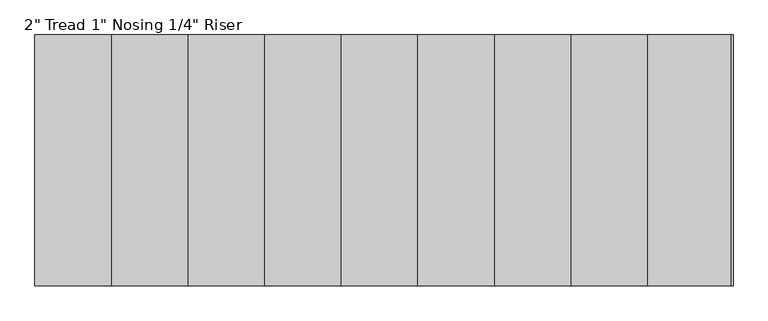
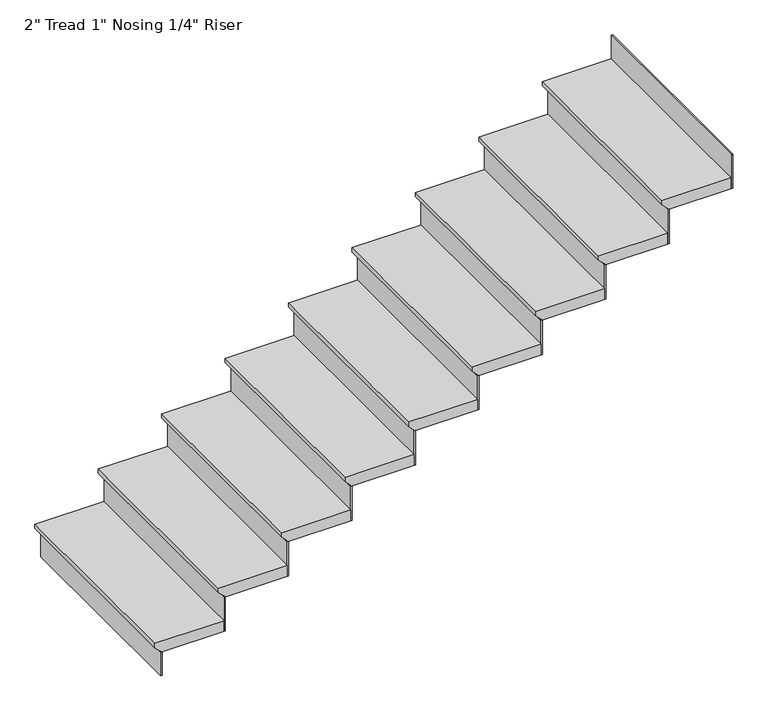
"""IFC4 building model written with IfcOpenShell, lengths in millimetres: stair flight geometry."""

from ifc_helpers import new_model, si_unit, origin, place, context, project, spatial, faceted_brep, source, transform, mapped, element, save


def stair_flight_228e22e8(model_context):
    return source(origin(), model_context, "Body", "Brep", [
        faceted_brep([(-1591.1154463, -4737.3544725, 9742.17), (-1591.1154463, -4737.3544725, 9761.22), (-1591.1154463, -3822.9544725, 9761.22), (-1591.1154463, -3822.9544725, 9742.17), (-1565.7154463, -4737.3544725, 9716.77), (-1565.7154463, -3822.9544725, 9716.77), (-1286.3154463, -4737.3544725, 9761.22), (-1286.3154463, -3822.9544725, 9761.22), (-1565.7154463, -3822.9544725, 9710.42), (-1286.3154463, -3822.9544725, 9710.42), (-1286.3154463, -4737.3544725, 9710.42), (-1565.7154463, -4737.3544725, 9710.42)], [[[0, 1, 2, 3]], [[4, 0, 3, 5]], [[2, 1, 6, 7]], [[8, 9, 10, 11]], [[2, 7, 9, 8, 5, 3]], [[8, 11, 4, 5]], [[6, 1, 0, 4, 11, 10]], [[7, 6, 10, 9]]]),
        faceted_brep([(-1565.7154463, -4737.3544725, 9710.42), (-1565.7154463, -4737.3544725, 9601.2), (-1559.3654463, -4737.3544725, 9601.2), (-1559.3654463, -4737.3544725, 9710.42), (-1565.7154463, -3822.9544725, 9710.42), (-1559.3654463, -3822.9544725, 9710.42), (-1559.3654463, -3822.9544725, 9601.2), (-1565.7154463, -3822.9544725, 9601.2)], [[[0, 1, 2, 3]], [[4, 5, 6, 7]], [[1, 0, 4, 7]], [[2, 1, 7, 6]], [[3, 2, 6, 5]], [[0, 3, 5, 4]]]),
        faceted_brep([(-1286.3154463, -4737.3544725, 9870.44), (-1286.3154463, -4737.3544725, 9710.42), (-1279.9654463, -4737.3544725, 9710.42), (-1279.9654463, -4737.3544725, 9870.44), (-1286.3154463, -3822.9544725, 9870.44), (-1279.9654463, -3822.9544725, 9870.44), (-1279.9654463, -3822.9544725, 9710.42), (-1286.3154463, -3822.9544725, 9710.42)], [[[0, 1, 2, 3]], [[4, 5, 6, 7]], [[1, 0, 4, 7]], [[2, 1, 7, 6]], [[3, 2, 6, 5]], [[0, 3, 5, 4]]]),
        faceted_brep([(-1311.7154463, -3822.9544725, 9921.24), (-1311.7154463, -4737.3544725, 9921.24), (-1006.9154463, -4737.3544725, 9921.24), (-1006.9154463, -3822.9544725, 9921.24), (-1286.3154463, -3822.9544725, 9870.44), (-1006.9154463, -3822.9544725, 9870.44), (-1006.9154463, -4737.3544725, 9870.44), (-1286.3154463, -4737.3544725, 9870.44), (-1286.3154463, -3822.9544725, 9876.79), (-1311.7154463, -3822.9544725, 9902.19), (-1286.3154463, -4737.3544725, 9876.79), (-1311.7154463, -4737.3544725, 9902.19)], [[[0, 1, 2, 3]], [[4, 5, 6, 7]], [[0, 3, 5, 4, 8, 9]], [[4, 7, 10, 8]], [[2, 1, 11, 10, 7, 6]], [[3, 2, 6, 5]], [[11, 1, 0, 9]], [[10, 11, 9, 8]]]),
        faceted_brep([(-1006.9154463, -4737.3544725, 10030.46), (-1006.9154463, -4737.3544725, 9870.44), (-1000.5654463, -4737.3544725, 9870.44), (-1000.5654463, -4737.3544725, 10030.46), (-1006.9154463, -3822.9544725, 10030.46), (-1000.5654463, -3822.9544725, 10030.46), (-1000.5654463, -3822.9544725, 9870.44), (-1006.9154463, -3822.9544725, 9870.44)], [[[0, 1, 2, 3]], [[4, 5, 6, 7]], [[1, 0, 4, 7]], [[2, 1, 7, 6]], [[3, 2, 6, 5]], [[0, 3, 5, 4]]]),
        faceted_brep([(-1032.3154463, -3822.9544725, 10081.26), (-1032.3154463, -4737.3544725, 10081.26), (-727.5154463, -4737.3544725, 10081.26), (-727.5154463, -3822.9544725, 10081.26), (-1006.9154463, -3822.9544725, 10030.46), (-727.5154463, -3822.9544725, 10030.46), (-727.5154463, -4737.3544725, 10030.46), (-1006.9154463, -4737.3544725, 10030.46), (-1006.9154463, -3822.9544725, 10036.81), (-1032.3154463, -3822.9544725, 10062.21), (-1006.9154463, -4737.3544725, 10036.81), (-1032.3154463, -4737.3544725, 10062.21)], [[[0, 1, 2, 3]], [[4, 5, 6, 7]], [[0, 3, 5, 4, 8, 9]], [[4, 7, 10, 8]], [[2, 1, 11, 10, 7, 6]], [[3, 2, 6, 5]], [[11, 1, 0, 9]], [[10, 11, 9, 8]]]),
        faceted_brep([(-727.5154463, -4737.3544725, 10190.48), (-727.5154463, -4737.3544725, 10030.46), (-721.1654463, -4737.3544725, 10030.46), (-721.1654463, -4737.3544725, 10190.48), (-727.5154463, -3822.9544725, 10190.48), (-721.1654463, -3822.9544725, 10190.48), (-721.1654463, -3822.9544725, 10030.46), (-727.5154463, -3822.9544725, 10030.46)], [[[0, 1, 2, 3]], [[4, 5, 6, 7]], [[1, 0, 4, 7]], [[2, 1, 7, 6]], [[3, 2, 6, 5]], [[0, 3, 5, 4]]]),
        faceted_brep([(-752.9154463, -3822.9544725, 10241.28), (-752.9154463, -4737.3544725, 10241.28), (-448.1154463, -4737.3544725, 10241.28), (-448.1154463, -3822.9544725, 10241.28), (-727.5154463, -3822.9544725, 10190.48), (-448.1154463, -3822.9544725, 10190.48), (-448.1154463, -4737.3544725, 10190.48), (-727.5154463, -4737.3544725, 10190.48), (-727.5154463, -3822.9544725, 10196.83), (-752.9154463, -3822.9544725, 10222.23), (-727.5154463, -4737.3544725, 10196.83), (-752.9154463, -4737.3544725, 10222.23)], [[[0, 1, 2, 3]], [[4, 5, 6, 7]], [[0, 3, 5, 4, 8, 9]], [[4, 7, 10, 8]], [[2, 1, 11, 10, 7, 6]], [[3, 2, 6, 5]], [[11, 1, 0, 9]], [[10, 11, 9, 8]]]),
        faceted_brep([(-448.1154463, -4737.3544725, 10350.5), (-448.1154463, -4737.3544725, 10190.48), (-441.7654463, -4737.3544725, 10190.48), (-441.7654463, -4737.3544725, 10350.5), (-448.1154463, -3822.9544725, 10350.5), (-441.7654463, -3822.9544725, 10350.5), (-441.7654463, -3822.9544725, 10190.48), (-448.1154463, -3822.9544725, 10190.48)], [[[0, 1, 2, 3]], [[4, 5, 6, 7]], [[1, 0, 4, 7]], [[2, 1, 7, 6]], [[3, 2, 6, 5]], [[0, 3, 5, 4]]]),
        faceted_brep([(-473.5154463, -3822.9544725, 10401.3), (-473.5154463, -4737.3544725, 10401.3), (-168.7154463, -4737.3544725, 10401.3), (-168.7154463, -3822.9544725, 10401.3), (-448.1154463, -3822.9544725, 10350.5), (-168.7154463, -3822.9544725, 10350.5), (-168.7154463, -4737.3544725, 10350.5), (-448.1154463, -4737.3544725, 10350.5), (-448.1154463, -3822.9544725, 10356.85), (-473.5154463, -3822.9544725, 10382.25), (-448.1154463, -4737.3544725, 10356.85), (-473.5154463, -4737.3544725, 10382.25)], [[[0, 1, 2, 3]], [[4, 5, 6, 7]], [[0, 3, 5, 4, 8, 9]], [[4, 7, 10, 8]], [[2, 1, 11, 10, 7, 6]], [[3, 2, 6, 5]], [[11, 1, 0, 9]], [[10, 11, 9, 8]]]),
        faceted_brep([(-168.7154463, -4737.3544725, 10510.52), (-168.7154463, -4737.3544725, 10350.5), (-162.3654463, -4737.3544725, 10350.5), (-162.3654463, -4737.3544725, 10510.52), (-168.7154463, -3822.9544725, 10510.52), (-162.3654463, -3822.9544725, 10510.52), (-162.3654463, -3822.9544725, 10350.5), (-168.7154463, -3822.9544725, 10350.5)], [[[0, 1, 2, 3]], [[4, 5, 6, 7]], [[1, 0, 4, 7]], [[2, 1, 7, 6]], [[3, 2, 6, 5]], [[0, 3, 5, 4]]]),
        faceted_brep([(-194.1154463, -3822.9544725, 10561.32), (-194.1154463, -4737.3544725, 10561.32), (110.6845537, -4737.3544725, 10561.32), (110.6845537, -3822.9544725, 10561.32), (-168.7154463, -3822.9544725, 10510.52), (110.6845537, -3822.9544725, 10510.52), (110.6845537, -4737.3544725, 10510.52), (-168.7154463, -4737.3544725, 10510.52), (-168.7154463, -3822.9544725, 10516.87), (-194.1154463, -3822.9544725, 10542.27), (-168.7154463, -4737.3544725, 10516.87), (-194.1154463, -4737.3544725, 10542.27)], [[[0, 1, 2, 3]], [[4, 5, 6, 7]], [[0, 3, 5, 4, 8, 9]], [[4, 7, 10, 8]], [[2, 1, 11, 10, 7, 6]], [[3, 2, 6, 5]], [[11, 1, 0, 9]], [[10, 11, 9, 8]]]),
        faceted_brep([(110.6845537, -4737.3544725, 10670.54), (110.6845537, -4737.3544725, 10510.52), (117.0345537, -4737.3544725, 10510.52), (117.0345537, -4737.3544725, 10670.54), (110.6845537, -3822.9544725, 10670.54), (117.0345537, -3822.9544725, 10670.54), (117.0345537, -3822.9544725, 10510.52), (110.6845537, -3822.9544725, 10510.52)], [[[0, 1, 2, 3]], [[4, 5, 6, 7]], [[1, 0, 4, 7]], [[2, 1, 7, 6]], [[3, 2, 6, 5]], [[0, 3, 5, 4]]]),
        faceted_brep([(85.2845537, -3822.9544725, 10721.34), (85.2845537, -4737.3544725, 10721.34), (390.0845537, -4737.3544725, 10721.34), (390.0845537, -3822.9544725, 10721.34), (110.6845537, -3822.9544725, 10670.54), (390.0845537, -3822.9544725, 10670.54), (390.0845537, -4737.3544725, 10670.54), (110.6845537, -4737.3544725, 10670.54), (110.6845537, -3822.9544725, 10676.89), (85.2845537, -3822.9544725, 10702.29), (110.6845537, -4737.3544725, 10676.89), (85.2845537, -4737.3544725, 10702.29)], [[[0, 1, 2, 3]], [[4, 5, 6, 7]], [[0, 3, 5, 4, 8, 9]], [[4, 7, 10, 8]], [[2, 1, 11, 10, 7, 6]], [[3, 2, 6, 5]], [[11, 1, 0, 9]], [[10, 11, 9, 8]]]),
        faceted_brep([(390.0845537, -4737.3544725, 10830.56), (390.0845537, -4737.3544725, 10670.54), (396.4345537, -4737.3544725, 10670.54), (396.4345537, -4737.3544725, 10830.56), (390.0845537, -3822.9544725, 10830.56), (396.4345537, -3822.9544725, 10830.56), (396.4345537, -3822.9544725, 10670.54), (390.0845537, -3822.9544725, 10670.54)], [[[0, 1, 2, 3]], [[4, 5, 6, 7]], [[1, 0, 4, 7]], [[2, 1, 7, 6]], [[3, 2, 6, 5]], [[0, 3, 5, 4]]]),
        faceted_brep([(364.6845537, -3822.9544725, 10881.36), (364.6845537, -4737.3544725, 10881.36), (669.4845537, -4737.3544725, 10881.36), (669.4845537, -3822.9544725, 10881.36), (390.0845537, -3822.9544725, 10830.56), (669.4845537, -3822.9544725, 10830.56), (669.4845537, -4737.3544725, 10830.56), (390.0845537, -4737.3544725, 10830.56), (390.0845537, -3822.9544725, 10836.91), (364.6845537, -3822.9544725, 10862.31), (390.0845537, -4737.3544725, 10836.91), (364.6845537, -4737.3544725, 10862.31)], [[[0, 1, 2, 3]], [[4, 5, 6, 7]], [[0, 3, 5, 4, 8, 9]], [[4, 7, 10, 8]], [[2, 1, 11, 10, 7, 6]], [[3, 2, 6, 5]], [[11, 1, 0, 9]], [[10, 11, 9, 8]]]),
        faceted_brep([(948.8845537, -4737.3544725, 11150.6), (948.8845537, -4737.3544725, 10990.58), (955.2345537, -4737.3544725, 10990.58), (955.2345537, -4737.3544725, 11150.6), (948.8845537, -3822.9544725, 11150.6), (955.2345537, -3822.9544725, 11150.6), (955.2345537, -3822.9544725, 10990.58), (948.8845537, -3822.9544725, 10990.58)], [[[0, 1, 2, 3]], [[4, 5, 6, 7]], [[1, 0, 4, 7]], [[2, 1, 7, 6]], [[3, 2, 6, 5]], [[0, 3, 5, 4]]]),
        faceted_brep([(669.4845537, -4737.3544725, 10990.58), (669.4845537, -4737.3544725, 10830.56), (675.8345537, -4737.3544725, 10830.56), (675.8345537, -4737.3544725, 10990.58), (669.4845537, -3822.9544725, 10990.58), (675.8345537, -3822.9544725, 10990.58), (675.8345537, -3822.9544725, 10830.56), (669.4845537, -3822.9544725, 10830.56)], [[[0, 1, 2, 3]], [[4, 5, 6, 7]], [[1, 0, 4, 7]], [[2, 1, 7, 6]], [[3, 2, 6, 5]], [[0, 3, 5, 4]]]),
        faceted_brep([(948.8845537, -3822.9544725, 11041.38), (923.4845537, -3822.9544725, 11041.38), (644.0845537, -3822.9544725, 11041.38), (644.0845537, -4737.3544725, 11041.38), (948.8845537, -4737.3544725, 11041.38), (923.4845537, -3822.9544725, 10990.58), (948.8845537, -3822.9544725, 10990.58), (948.8845537, -4737.3544725, 10990.58), (669.4845537, -4737.3544725, 10990.58), (669.4845537, -3822.9544725, 10990.58), (669.4845537, -3822.9544725, 10996.93), (644.0845537, -3822.9544725, 11022.33), (669.4845537, -4737.3544725, 10996.93), (644.0845537, -4737.3544725, 11022.33)], [[[0, 1, 2, 3, 4]], [[5, 6, 7, 8, 9]], [[1, 0, 6, 5]], [[2, 1, 5, 9, 10, 11]], [[9, 8, 12, 10]], [[4, 3, 13, 12, 8, 7]], [[0, 4, 7, 6]], [[13, 3, 2, 11]], [[12, 13, 11, 10]]]),
    ])


if __name__ == "__main__":
    model = new_model("IFC4")
    model_context = context("Model", 3, world=origin())
    ifc_project = project(units=[si_unit("LENGTHUNIT", "METRE", prefix="MILLI")], contexts=[model_context])
    site = spatial("IfcSite", under=ifc_project)
    building = spatial("IfcBuilding", under=site)
    placement = place(None, origin())
    stair_flight_shape = stair_flight_228e22e8(model_context)
    element("IfcStairFlight", 1, ObjectType="2\" Tread 1\" Nosing 1/4\" Riser", at=placement, inside=building, context=model_context, shape_type="MappedRepresentation", body=[
        mapped(stair_flight_shape, transform((0.0, 0.0, 0.0), x_axis=(1.0, 0.0, 0.0), y_axis=(0.0, 1.0, 0.0), z_axis=(0.0, 0.0, 1.0))),
    ])
    save(model, "model.ifc")
